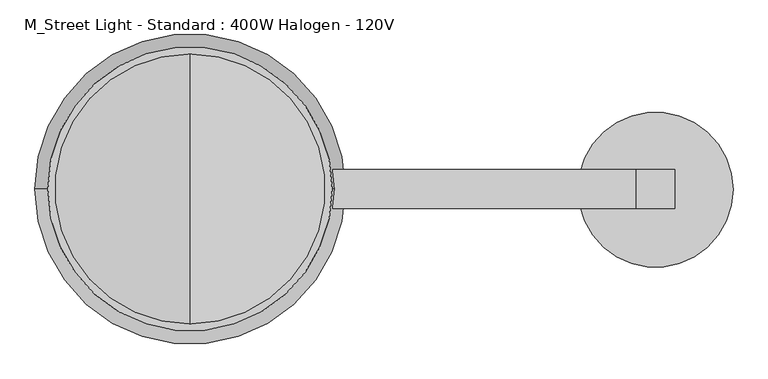
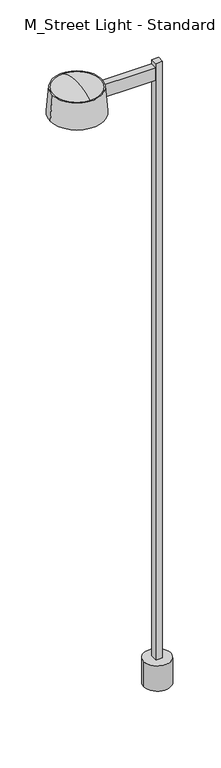
"""IFC4 building model written with IfcOpenShell, lengths in millimetres: light fixture geometry, M_Street Light - Standard : 400W Halogen - 120V."""

from ifc_helpers import new_model, si_unit, point, frame, origin, origin_with_axes, origin_2d, place, context, project, spatial, polyline, circle_curve, ellipse_curve, trimmed, segment, composite_curve, outline, extrude, source, transform, mapped, element, save
from ifc_brep_helpers import plane_surface, revolved_surface, advanced_brep


def m_street_light_standard_400w_halogen_120v_204dbcbb(model_context):
    return source(origin(), model_context, "Body", "SolidModel", [
        extrude(outline(composite_curve([segment(trimmed(circle_curve(origin_2d(), 152.4), [point((-152.4, 0.0))], [point((152.4, 0.0))], False, "CARTESIAN"), True, "CONTINUOUS"), segment(trimmed(circle_curve(origin_2d(), 152.4), [point((152.4, 0.0))], [point((-152.4, 0.0))], False, "CARTESIAN"), True, "CONTINUOUS")], self_intersect=False)), origin_with_axes(), (0.0, 0.0, 1.0), 304.8),
        extrude(outline(polyline([(38.1, 38.1), (38.1, -38.1), (-38.1, -38.1), (-38.1, 38.1), (38.1, 38.1)])), frame((0.0, 0.0, 304.8), z_axis=(0.0, 0.0, 1.0), x_axis=(1.0, 0.0, 0.0)), (0.0, 0.0, 1.0), 7195.2),
        extrude(outline(polyline([(-914.4, 38.1), (-38.1, 38.1), (-38.1, -38.1), (-914.4, -38.1), (-914.4, 38.1)])), frame((0.0, 0.0, 7296.8), z_axis=(0.0, 0.0, 1.0), x_axis=(1.0, 0.0, 0.0)), (0.0, 0.0, 1.0), 152.4),
        advanced_brep(
        [(-1193.8, 0.0, 7500.0), (-635.0, 0.0, 7500.0), (-1219.2, 0.0, 7195.2), (-609.6, 0.0, 7195.2)],
        [
            (0, 1, circle_curve(frame((-914.4, 0.0, 7500.0), z_axis=(0.0, 0.0, 1.0), x_axis=(-1.0, 0.0, 0.0)), 279.4)),
            (1, 0, circle_curve(frame((-914.4, 0.0, 7500.0), z_axis=(0.0, 0.0, 1.0), x_axis=(1.0, 0.0, 0.0)), 279.4)),
            (2, 3, circle_curve(frame((-914.4, 0.0, 7195.2), z_axis=(0.0, 0.0, -1.0), x_axis=(1.0, 0.0, 0.0)), 304.8)),
            (3, 2, circle_curve(frame((-914.4, 0.0, 7195.2), z_axis=(0.0, 0.0, -1.0), x_axis=(-1.0, 0.0, 0.0)), 304.8)),
            (3, 1),
            (0, 2),
        ],
        [
            plane_surface(frame((-914.4, 0.0, 7500.0), z_axis=(0.0, 0.0, 1.0), x_axis=(0.0, -1.0, 0.0))),
            plane_surface(frame((-914.4, 0.0, 7195.2), z_axis=(0.0, 0.0, -1.0), x_axis=(0.0, -1.0, 0.0))),
            revolved_surface(polyline([(-1193.8, 0.0, 7500.0), (-1219.2, 0.0, 7195.2)]), (-914.4, 0.0, 10852.8), (0.0, 0.0, -1.0)),
            revolved_surface(polyline([(-635.0, 0.0, 7500.0), (-609.6, 0.0, 7195.2)]), (-914.4, 0.0, 10852.8), (0.0, 0.0, -1.0)),
        ],
        [
            (0, [[1, 2]]),
            (1, [[3, 4]]),
            (2, [[-4, 5, -1, 6]]),
            (3, [[-3, -6, -2, -5]]),
        ],
    ),
        advanced_brep(
        [(-914.4, -266.7, 7500.0), (-914.4, 266.7, 7500.0), (-914.4, 0.0, 7571.4620496), (-914.4, -228.6332063, 7500.0), (-914.4, 228.6332063, 7500.0), (-914.4, 0.0, 7558.7620496)],
        [
            (0, 1, circle_curve(frame((-914.4, 0.0, 7500.0), z_axis=(0.0, 0.0, 1.0), x_axis=(0.0, 1.0, 0.0)), 266.7)),
            (1, 2, circle_curve(frame((-914.4, -28.9924067, 6929.8609147), z_axis=(1.0, 0.0, 0.0), x_axis=(0.0, 0.0, 1.0)), 642.2558493)),
            (2, 0, circle_curve(frame((-914.4, 28.9924067, 6929.8609147), z_axis=(1.0, 0.0, 0.0), x_axis=(0.0, 0.0, 1.0)), 642.2558493)),
            (1, 0, circle_curve(frame((-914.4, 0.0, 7500.0), z_axis=(0.0, 0.0, 1.0), x_axis=(0.0, 1.0, 0.0)), 266.7)),
            (3, 4, circle_curve(frame((-914.4, 0.0, 7500.0), z_axis=(0.0, 0.0, 1.0), x_axis=(0.0, 1.0, 0.0)), 228.6332063)),
            (4, 1),
            (0, 3),
            (4, 3, circle_curve(frame((-914.4, 0.0, 7500.0), z_axis=(0.0, 0.0, 1.0), x_axis=(0.0, 1.0, 0.0)), 228.6332063)),
            (5, 4),
            (3, 5),
        ],
        [
            revolved_surface(trimmed(ellipse_curve(frame((-914.4, -28.9924067, 6929.8609147), z_axis=(-1.0, 0.0, 0.0), x_axis=(0.0, 0.0, 1.0)), 642.2558493, 642.2558493), [point((-914.4, 0.0, 7571.4620496))], [point((-914.4, 266.7, 7500.0))], True, "CARTESIAN"), (-914.4, 0.0, 7423.8), (0.0, 0.0, -1.0)),
            plane_surface(frame((-914.4, 0.0, 7500.0), z_axis=(0.0, 0.0, -1.0), x_axis=(0.0, 1.0, 0.0))),
            revolved_surface(polyline([(-914.4, 228.6332063, 7500.0), (-914.4, 0.0, 7558.7620496)]), (-914.4, 0.0, 7423.8), (0.0, 0.0, -1.0)),
        ],
        [
            (0, [[1, 2, 3]]),
            (0, [[4, -3, -2]]),
            (1, [[5, 6, -1, 7]]),
            (1, [[8, -7, -4, -6]]),
            (2, [[9, -5, 10]]),
            (2, [[-10, -8, -9]]),
        ],
    ),
        advanced_brep(
        [(-914.4, -228.6332063, 7195.2), (-914.4, 228.6332063, 7195.2), (-914.4, 0.0, 7136.4379504), (-914.4, -266.7, 7195.2), (-914.4, 266.7, 7195.2), (-914.4, 0.0, 7123.7379504)],
        [
            (0, 1, circle_curve(frame((-914.4, 0.0, 7195.2), z_axis=(0.0, 0.0, 1.0), x_axis=(0.0, 1.0, 0.0)), 228.6332063)),
            (1, 2),
            (2, 0),
            (1, 0, circle_curve(frame((-914.4, 0.0, 7195.2), z_axis=(0.0, 0.0, 1.0), x_axis=(0.0, 1.0, 0.0)), 228.6332063)),
            (3, 4, circle_curve(frame((-914.4, 0.0, 7195.2), z_axis=(0.0, 0.0, 1.0), x_axis=(0.0, 1.0, 0.0)), 266.7)),
            (4, 1),
            (0, 3),
            (4, 3, circle_curve(frame((-914.4, 0.0, 7195.2), z_axis=(0.0, 0.0, 1.0), x_axis=(0.0, 1.0, 0.0)), 266.7)),
            (5, 4, circle_curve(frame((-914.4, -28.9924067, 7765.3390853), z_axis=(1.0, 0.0, 0.0), x_axis=(0.0, 0.0, -1.0)), 642.2558493)),
            (3, 5, circle_curve(frame((-914.4, 28.9924067, 7765.3390853), z_axis=(1.0, 0.0, 0.0), x_axis=(0.0, 0.0, -1.0)), 642.2558493)),
        ],
        [
            revolved_surface(polyline([(-914.4, 0.0, 7136.4379504), (-914.4, 228.6332063, 7195.2)]), (-914.4, 0.0, 7271.4), (0.0, 0.0, -1.0)),
            plane_surface(frame((-914.4, 0.0, 7195.2), z_axis=(0.0, 0.0, 1.0), x_axis=(0.0, 1.0, 0.0))),
            revolved_surface(trimmed(ellipse_curve(frame((-914.4, -28.9924067, 7765.3390853), z_axis=(-1.0, 0.0, 0.0), x_axis=(0.0, 0.0, -1.0)), 642.2558493, 642.2558493), [point((-914.4, 266.7, 7195.2))], [point((-914.4, 0.0, 7123.7379504))], True, "CARTESIAN"), (-914.4, 0.0, 7271.4), (0.0, 0.0, -1.0)),
        ],
        [
            (0, [[1, 2, 3]]),
            (0, [[4, -3, -2]]),
            (1, [[5, 6, -1, 7]]),
            (1, [[8, -7, -4, -6]]),
            (2, [[9, -5, 10]]),
            (2, [[-10, -8, -9]]),
        ],
    ),
    ])


if __name__ == "__main__":
    model = new_model("IFC4")
    model_context = context("Model", 3, world=origin())
    ifc_project = project(units=[si_unit("LENGTHUNIT", "METRE", prefix="MILLI")], contexts=[model_context])
    site = spatial("IfcSite", under=ifc_project)
    building = spatial("IfcBuilding", under=site)
    placement = place(None, origin())
    m_street_light_standard_400w_halogen_120v_shape = m_street_light_standard_400w_halogen_120v_204dbcbb(model_context)
    element("IfcLightFixture", 1, ObjectType="M_Street Light - Standard : 400W Halogen - 120V", at=placement, inside=building, context=model_context, shape_type="MappedRepresentation", body=[
        mapped(m_street_light_standard_400w_halogen_120v_shape, transform((0.0, 0.0, 0.0), x_axis=(1.0, 0.0, 0.0), y_axis=(0.0, 1.0, 0.0), z_axis=(0.0, 0.0, 1.0))),
    ])
    save(model, "model.ifc")

# Revit data of these elements
# Type "M_Street Light - Standard : 400W Halogen - 120V"
#   Photometric Web File = "SLS1T3.ies"
#   Lamp = "T-3"
#   Wattage Comments = "400"
#   Wattage = 800 W
#   built-in parameter 1150110 = 2 (stored number, unit not read)
#   built-in parameter 1114217 = 4 (stored number, unit not read)
#   built-in parameter 1150109 = 2 (stored number, unit not read)
#   built-in parameter 1150113 = 1 (stored number, unit not read)
#   Tilt Angle = -90.00°
#   built-in parameter 1150115 = 1 (stored number, unit not read)
#   built-in parameter 1150105 = 6366.2 (stored number, unit not read)
#   built-in parameter 1150112 = 1 (stored number, unit not read)
#   built-in parameter 1150114 = 1 (stored number, unit not read)
#   built-in parameter 1150107 = 6500 (stored number, unit not read)
#   built-in parameter 1150106 = 63.662 (stored number, unit not read)
#   Height = 24' - 7.27559"
#   Lumens = 80000 lm
#   built-in parameter 1150104 = 9.2903 (stored number, unit not read)
#   Voltage = 120 V
#   built-in parameter 1114218 = 1 (stored number, unit not read)
#   built-in parameter 1150133 = 10 (stored number, unit not read)
#   Apparent Load = 400 VA
#   built-in parameter 1150134 = 1
#   built-in parameter 1150137 = 1
#   Color Filter = 16777215
#   Number of poles = 1
#   Stand Material = Steel, Paint Finish, Dark Gray, Matte
#   Shade Material = Steel, Paint Finish, Dark Gray, Matte
#   Load Classification = Lighting - Exterior
#   Diffuser Material = Glass, Frosted
#   Dimming Lamp Color Temperature Shift = (empty or 0)
#   Default Elevation = 0
# Element 1 (IfcLightFixture, "M_Street Light - Standard : 400W Halogen - 120V")
#   Materials on its faces: "Steel, Paint Finish, Dark Gray, Matte", "Glass, Frosted"
# Materials
#   "Steel, Paint Finish, Dark Gray, Matte": class "Metal", colour RGB 98 98 98, transparency 0, Description = "Steel, paint finish, dark gray, matte", Cost = 0
#   "Glass, Frosted": class "Glass", colour RGB 250 244 225, transparency 0.55, Description = "physical material", Cost = 0
